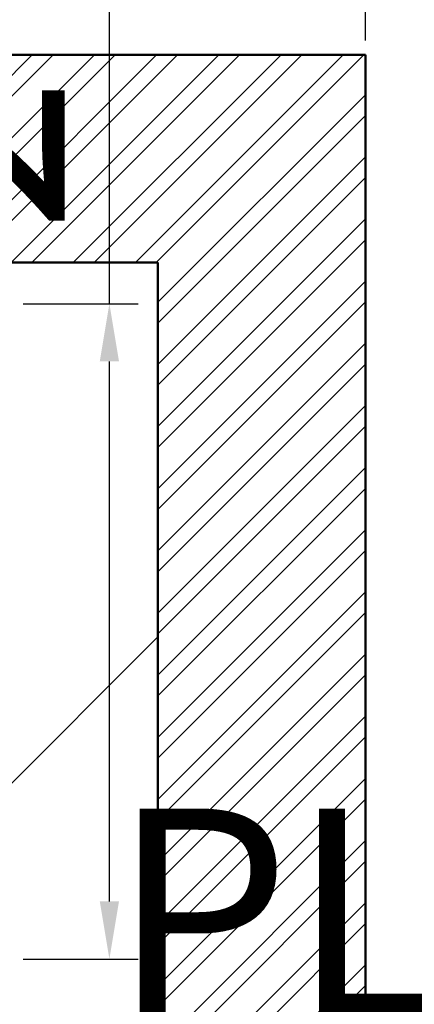
# Model space of a CAD drawing. Units: inches. Extents: x 3590 to 5167, y 65 to 1917.
# Tile 98 of 100: x 5065 to 5082, y 1765 to 1808. Entities that reach past the tile are written whole.
import ezdxf

# ---------------------------------------------------------------- set-up
doc = ezdxf.new("R2010")
doc.units = ezdxf.units.IN
for name, color, linetype, lineweight in [('A-ANNO-DIMS', 2, 'Continuous', 18), ('A-FLOR-PATT', 8, 'Continuous', 13), ('A-WALL', 7, 'Continuous', 50), ('A-WALL-PATT', 251, 'Continuous', 13)]:
    doc.layers.add(name, color=color, linetype=linetype, lineweight=lineweight)
doc.styles.get("Standard").update_dxf_attribs({"font": 'arial.ttf'})
doc.dimstyles.new('ISO-25', dxfattribs={"dimtxt": 9, "dimasz": 2.5, "dimexe": 1.25, "dimexo": 0.625, "dimtad": 1, "dimdec": 1, "dimlunit": 3, "dimtxsty": 'Standard', "dimcen": 2.5, "dimadec": 0, "dimazin": 0, "dimtfac": 1, "dimtdec": 1, "dimtmove": 0, "dimatfit": 3, "dimfxl": 1, "dimarcsym": 0})

# ---------------------------------------------------------------- blocks, each defined once
blk = doc.blocks.new('*D101')
at = {"layer": 'A-ANNO-DIMS', "color": 0, "lineweight": -2, "transparency": 16777216}
for p, q in [((4420.274, 1806.624), (4420.274, 1818.615)), ((5080.274, 1806.624), (5080.274, 1818.615)), ((4422.774, 1817.365), (5077.774, 1817.365))]:
    blk.add_line(p, q, dxfattribs=at)
at = {"layer": 'A-ANNO-DIMS', "color": 0, "transparency": 16777216}
for points in [[(4422.774, 1817.781), (4422.774, 1816.948), (4420.274, 1817.365)], [(5077.774, 1817.781), (5077.774, 1816.948), (5080.274, 1817.365)]]:
    blk.add_solid(points, dxfattribs=at)
at = {"layer": 'Defpoints', "color": 0, "transparency": 16777216}
for p in [(5080.274, 1817.365), (4420.274, 1805.999), (5080.274, 1805.999)]:
    blk.add_point(p, dxfattribs=at)
at = {"layer": 'A-ANNO-DIMS', "color": 0, "transparency": 16777216, "insert": (4750.274, 1822.566), "char_height": 9, "attachment_point": 5}
blk.add_mtext("55'", dxfattribs=at)
blk = doc.blocks.new('*D322')
at = {"layer": 'A-ANNO-DIMS', "color": 0, "lineweight": -2, "transparency": 16777216}
for p, q in [((5035.744, 1766.184), (5035.744, 1761.199)), ((5064.812, 1766.184), (5064.812, 1761.199)), ((5038.244, 1762.449), (5062.312, 1762.449)), ((5064.812, 1762.449), (5166.991, 1762.449))]:
    blk.add_line(p, q, dxfattribs=at)
at = {"layer": 'A-ANNO-DIMS', "color": 0, "transparency": 16777216}
for points in [[(5038.244, 1762.866), (5038.244, 1762.032), (5035.744, 1762.449)], [(5062.312, 1762.866), (5062.312, 1762.032), (5064.812, 1762.449)]]:
    blk.add_solid(points, dxfattribs=at)
at = {"layer": 'Defpoints', "color": 0, "transparency": 16777216}
for p in [(5035.744, 1766.809), (5064.812, 1766.809), (5064.812, 1762.449)]:
    blk.add_point(p, dxfattribs=at)
at = {"layer": 'A-ANNO-DIMS', "color": 0, "transparency": 16777216, "insert": (5117.152, 1767.669), "char_height": 9, "attachment_point": 5}
blk.add_mtext('PLANT 2\'-5" TYP.', dxfattribs=at)
blk = doc.blocks.new('*D323')
at = {"layer": 'A-ANNO-DIMS', "color": 0, "lineweight": -2, "transparency": 16777216}
for p, q in [((5069.172, 1795.216), (5069.172, 1874.95)), ((5065.437, 1795.216), (5070.422, 1795.216)), ((5069.172, 1769.309), (5069.172, 1792.716)), ((5065.437, 1766.809), (5070.422, 1766.809))]:
    blk.add_line(p, q, dxfattribs=at)
at = {"layer": 'A-ANNO-DIMS', "color": 0, "transparency": 16777216}
for points in [[(5068.756, 1792.716), (5069.589, 1792.716), (5069.172, 1795.216)], [(5068.756, 1769.309), (5069.589, 1769.309), (5069.172, 1766.809)]]:
    blk.add_solid(points, dxfattribs=at)
at = {"layer": 'Defpoints', "color": 0, "transparency": 16777216}
for p in [(5064.812, 1795.216), (5069.172, 1795.216), (5064.812, 1766.809)]:
    blk.add_point(p, dxfattribs=at)
at = {"layer": 'A-ANNO-DIMS', "color": 0, "transparency": 16777216, "insert": (5063.894, 1836.333), "char_height": 9, "attachment_point": 5, "rotation": 90}
blk.add_mtext('2\'-4 1/2" TYP.', dxfattribs=at)

msp = doc.modelspace()

# ---------------------------------------------------------------- hatches: boundary and pattern name
at = {"layer": 'A-FLOR-PATT', "transparency": 33554687}
h = msp.add_hatch(dxfattribs=at)
h.set_pattern_fill('AR-HBONE', color=256, scale=0.2)
h.set_pattern_definition([(45, (-588.972, 0), (0, 28.73682), [60.96, -20.32]), (135, (-574.604, 14.368), (3e-15, 28.73682), [60.96, -20.32])])
h.paths.add_polyline_path([(5071.274, 1796.999), (4933.274, 1796.999), (4933.274, 1753.999), (4962.774, 1753.999, -0.414214), (4928.774, 1719.999), (4933.274, 1718.999), (4933.274, 1334.999), (5071.274, 1334.999)])
h.paths.add_polyline_path([(4951.78, 1521.077), (4951.715, 1521.04), (4951.563, 1520.895)], flags=16)
h.paths.add_polyline_path([(4952.267, 1521.376), (4952.198, 1521.371), (4952.198, 1521.356)], flags=0)
h.paths.add_polyline_path([(4967.051, 1529.728), (4965.231, 1528.694), (4963.411, 1527.714), (4961.756, 1526.851), (4963.589, 1527.449), (4964.036, 1527.478), (4962.975, 1527.249), (4961.76, 1526.852), (4959.792, 1525.834), (4958.005, 1524.895), (4956.24, 1523.93), (4954.504, 1522.919), (4954.129, 1522.682), (4953.361, 1521.997), (4953.366, 1521.998), (4953.605, 1522.064), (4955.106, 1522.761), (4956.921, 1523.434), (4958.678, 1523.915), (4960.358, 1524.2), (4961.945, 1524.286), (4964.171, 1524.108), (4965.958, 1523.309), (4963.863, 1522.976), (4965.187, 1522.499), (4963.366, 1522.497), (4961.545, 1522.487), (4959.764, 1522.461), (4958.304, 1522.419), (4957.974, 1522.388), (4956.307, 1522.232), (4954.718, 1522.071), (4953.251, 1521.899), (4953.525, 1521.623), (4954.331, 1521.379), (4956.243, 1521.23), (4958.039, 1520.93), (4959.684, 1520.483), (4961.16, 1519.896), (4963.107, 1518.8), (4964.393, 1517.325), (4962.973, 1517.726), (4964.558, 1516.661), (4965.407, 1515.708), (4963.507, 1516.322), (4961.68, 1517.005), (4959.935, 1517.745), (4958.282, 1518.528), (4956.732, 1519.343), (4955.295, 1520.175), (4954.672, 1520.572), (4954.513, 1520.627), (4955.658, 1519.318), (4956.703, 1517.982), (4957.644, 1516.647), (4958.485, 1515.334), (4959.55, 1513.524), (4960.438, 1511.769), (4958.841, 1513.62), (4957.452, 1515.325), (4955.819, 1517.459), (4956.665, 1515.448), (4957.111, 1513.923), (4957.447, 1511.714), (4957.076, 1509.793), (4956.538, 1511.11), (4955.992, 1512.569), (4955.444, 1514.125), (4954.898, 1515.735), (4954.357, 1517.356), (4953.824, 1518.943), (4953.305, 1520.452), (4953.065, 1521.116), (4952.971, 1521.146), (4952.949, 1521.086), (4952.73, 1520.199), (4953.37, 1518.024), (4953.757, 1516.373), (4954.051, 1514.765), (4954.264, 1513.221), (4954.471, 1511.131), (4954.497, 1510.402), (4954.409, 1511.76), (4954.264, 1513.221), (4954.051, 1514.765), (4953.757, 1516.373), (4953.37, 1518.024), (4952.877, 1519.698), (4952.716, 1520.141), (4952.533, 1519.059), (4952.374, 1517.789), (4952.219, 1516.312), (4952.046, 1514.6), (4951.833, 1512.626), (4951.557, 1510.363), (4951.203, 1512.168), (4950.852, 1514.339), (4950.985, 1516.376), (4951.66, 1518.286), (4952.593, 1520.481), (4952.357, 1521.13), (4951.855, 1520.328), (4950.839, 1518.908), (4949.777, 1517.587), (4948.916, 1516.617), (4948.111, 1515.256), (4947.089, 1513.554), (4945.889, 1511.615), (4946.326, 1513.402), (4946.562, 1514.249), (4945.528, 1513.327), (4944.581, 1512.531), (4946.018, 1514.508), (4947.204, 1516.048), (4947.893, 1517.313), (4949.307, 1518.764), (4950.414, 1519.767), (4950.451, 1519.806), (4952.267, 1521.376), (4951.645, 1521.493), (4950.404, 1521.18), (4948.044, 1520.359), (4946.119, 1519.452), (4944.572, 1518.475), (4943.35, 1517.443), (4941.997, 1515.92), (4941.661, 1515.275), (4942.813, 1516.99), (4944.572, 1518.475), (4946.119, 1519.452), (4948.044, 1520.359), (4950.404, 1521.18), (4951.645, 1521.493), (4949.647, 1521.868), (4948.6, 1521.756), (4947.126, 1521.57), (4945.42, 1521.348), (4943.45, 1521.105), (4941.183, 1520.856), (4942.86, 1521.613), (4943.873, 1522.03), (4942.952, 1521.909), (4941.41, 1521.485), (4939.543, 1520.67), (4938.968, 1520.226), (4940.733, 1521.299), (4942.952, 1521.909), (4943.702, 1522.008), (4945.894, 1522.7), (4947.565, 1522.714), (4948.921, 1522.566), (4951.131, 1522.183), (4950.971, 1522.297), (4948.129, 1523.006), (4946.035, 1523.707), (4944.232, 1524.521), (4942.707, 1525.461), (4941.444, 1526.537), (4940.43, 1527.761), (4939.649, 1529.143), (4941.421, 1528.122), (4943.147, 1527.132), (4944.841, 1526.175), (4946.514, 1525.25), (4948.179, 1524.359), (4948.365, 1524.263), (4946.475, 1526.045), (4945.181, 1527.54), (4944.19, 1529.033), (4943.496, 1530.54), (4943.278, 1531.36), (4942.498, 1531.919), (4943.114, 1531.762), (4942.959, 1533.659), (4944.14, 1531.989), (4944.612, 1531.323), (4946.202, 1530.463), (4947.486, 1529.509), (4948.79, 1528.226), (4950.368, 1526.237), (4949.485, 1528.155), (4948.851, 1530.123), (4948.491, 1532.041), (4948.381, 1533.918), (4948.501, 1535.76), (4948.827, 1537.573), (4949.418, 1535.565), (4949.957, 1533.569), (4950.464, 1531.586), (4950.961, 1529.617), (4951.391, 1527.954), (4951.724, 1530.687), (4952.201, 1532.58), (4952.889, 1534.33), (4953.77, 1535.951), (4954.827, 1537.46), (4954.521, 1535.39), (4954.273, 1533.937), (4955.58, 1535.663), (4956.748, 1536.739), (4956.159, 1534.78), (4955.589, 1532.873), (4955.043, 1531.006), (4954.525, 1529.166), (4954.038, 1527.341), (4953.638, 1525.733), (4953.611, 1525.586), (4953.398, 1524.166), (4953.382, 1524.009), (4954.07, 1525.476), (4954.912, 1527.022), (4956.136, 1528.894), (4957.847, 1530.577), (4959.376, 1531.54), (4958.256, 1530.104), (4957.143, 1528.663), (4956.066, 1527.243), (4955.056, 1525.871), (4954.141, 1524.571), (4953.352, 1523.372), (4953.311, 1523.303), (4953.273, 1522.925), (4953.261, 1522.382), (4954.103, 1523.373), (4954.63, 1524.284), (4955.961, 1526.358), (4957.23, 1528.13), (4958.421, 1529.609), (4960.037, 1531.368), (4961.374, 1532.375), (4962.101, 1532.77), (4961.07, 1531.061), (4959.987, 1529.438), (4958.869, 1527.908), (4958.15, 1527.007), (4959.803, 1528.003), (4961.589, 1528.793), (4963.391, 1529.328), (4965.211, 1529.632)], flags=16)
h.paths.add_polyline_path([(4962.944, 1523.182), (4961.107, 1523.422), (4960.392, 1523.362), (4962.35, 1523.331)], flags=0)
h.paths.add_polyline_path([(5049.541, 1584.551), (5049.476, 1584.515), (5049.325, 1584.37)], flags=16)
h.paths.add_polyline_path([(5050.028, 1584.851), (5049.959, 1584.845), (5049.959, 1584.83)], flags=0)
h.paths.add_polyline_path([(5042.333, 1581.949), (5043.88, 1582.926), (5045.806, 1583.833), (5048.165, 1584.654), (5049.406, 1584.967), (5047.408, 1585.342), (5046.361, 1585.231), (5044.888, 1585.044), (5043.181, 1584.822), (5041.211, 1584.579), (5038.944, 1584.33), (5040.622, 1585.087), (5041.634, 1585.504), (5040.713, 1585.383), (5039.171, 1584.959), (5037.304, 1584.144), (5036.729, 1583.7), (5038.494, 1584.773), (5040.713, 1585.383), (5041.463, 1585.482), (5043.655, 1586.174), (5045.326, 1586.188), (5046.682, 1586.04), (5048.893, 1585.657), (5048.732, 1585.771), (5045.891, 1586.48), (5043.796, 1587.181), (5041.994, 1587.996), (5040.468, 1588.935), (5039.205, 1590.011), (5038.191, 1591.235), (5037.41, 1592.617), (5039.182, 1591.596), (5040.909, 1590.607), (5042.602, 1589.649), (5044.275, 1588.724), (5045.94, 1587.833), (5046.126, 1587.738), (5044.237, 1589.519), (5042.942, 1591.015), (5041.952, 1592.508), (5041.257, 1594.014), (5041.039, 1594.834), (5040.26, 1595.393), (5040.875, 1595.237), (5040.721, 1597.133), (5041.901, 1595.463), (5042.373, 1594.798), (5043.963, 1593.938), (5045.247, 1592.983), (5046.552, 1591.701), (5048.129, 1589.712), (5047.247, 1591.63), (5046.613, 1593.597), (5046.252, 1595.515), (5046.142, 1597.392), (5046.262, 1599.234), (5046.588, 1601.047), (5047.179, 1599.039), (5047.718, 1597.043), (5048.225, 1595.06), (5048.722, 1593.091), (5049.152, 1591.429), (5049.485, 1594.161), (5049.962, 1596.054), (5050.65, 1597.804), (5051.532, 1599.425), (5052.589, 1600.934), (5052.283, 1598.864), (5052.034, 1597.411), (5053.341, 1599.137), (5054.509, 1600.213), (5053.92, 1598.254), (5053.35, 1596.348), (5052.805, 1594.48), (5052.286, 1592.64), (5051.799, 1590.815), (5051.4, 1589.207), (5051.373, 1589.06), (5051.159, 1587.64), (5051.143, 1587.483), (5051.831, 1588.95), (5052.673, 1590.496), (5053.898, 1592.368), (5055.608, 1594.051), (5057.137, 1595.014), (5056.017, 1593.578), (5054.904, 1592.137), (5053.828, 1590.717), (5052.817, 1589.345), (5051.902, 1588.046), (5051.113, 1586.846), (5051.072, 1586.777), (5051.034, 1586.399), (5051.022, 1585.856), (5051.864, 1586.847), (5052.391, 1587.758), (5053.723, 1589.832), (5054.991, 1591.604), (5056.182, 1593.083), (5057.798, 1594.842), (5059.135, 1595.849), (5059.863, 1596.244), (5058.831, 1594.535), (5057.749, 1592.912), (5056.63, 1591.382), (5055.912, 1590.482), (5057.564, 1591.477), (5059.35, 1592.267), (5061.152, 1592.802), (5062.972, 1593.106), (5064.812, 1593.203), (5062.992, 1592.169), (5061.172, 1591.188), (5059.518, 1590.325), (5061.35, 1590.924), (5061.797, 1590.952), (5060.737, 1590.723), (5059.521, 1590.326), (5057.553, 1589.308), (5055.766, 1588.369), (5054.002, 1587.404), (5052.265, 1586.393), (5051.891, 1586.156), (5051.122, 1585.471), (5051.127, 1585.472), (5051.366, 1585.538), (5052.867, 1586.235), (5054.682, 1586.908), (5056.439, 1587.389), (5058.12, 1587.675), (5059.706, 1587.76), (5061.933, 1587.583), (5063.719, 1586.783), (5061.624, 1586.45), (5062.949, 1585.973), (5061.127, 1585.971), (5059.307, 1585.961), (5057.525, 1585.935), (5056.065, 1585.893), (5055.735, 1585.862), (5054.068, 1585.707), (5052.479, 1585.546), (5051.012, 1585.373), (5051.286, 1585.097), (5052.092, 1584.853), (5054.004, 1584.704), (5055.8, 1584.404), (5057.446, 1583.958), (5058.921, 1583.37), (5060.868, 1582.274), (5062.154, 1580.799), (5060.734, 1581.2), (5062.32, 1580.135), (5063.168, 1579.182), (5061.269, 1579.796), (5059.441, 1580.479), (5057.696, 1581.219), (5056.043, 1582.003), (5054.493, 1582.817), (5053.057, 1583.649), (5052.433, 1584.047), (5052.274, 1584.101), (5053.42, 1582.793), (5054.464, 1581.457), (5055.405, 1580.121), (5056.247, 1578.809), (5057.311, 1576.998), (5058.199, 1575.244), (5056.602, 1577.094), (5055.213, 1578.799), (5053.58, 1580.933), (5054.427, 1578.922), (5054.872, 1577.397), (5055.208, 1575.189), (5054.838, 1573.267), (5054.299, 1574.584), (5053.754, 1576.043), (5053.206, 1577.599), (5052.659, 1579.209), (5052.118, 1580.83), (5051.585, 1582.417), (5051.066, 1583.927), (5050.826, 1584.59), (5050.733, 1584.62), (5050.711, 1584.561), (5050.491, 1583.673), (5051.131, 1581.498), (5051.518, 1579.847), (5051.813, 1578.24), (5052.026, 1576.695), (5052.233, 1574.605), (5052.258, 1573.876), (5052.17, 1575.234), (5052.026, 1576.695), (5051.813, 1578.24), (5051.518, 1579.847), (5051.131, 1581.498), (5050.638, 1583.172), (5050.477, 1583.615), (5050.294, 1582.533), (5050.136, 1581.263), (5049.981, 1579.786), (5049.807, 1578.074), (5049.594, 1576.1), (5049.318, 1573.837), (5048.965, 1575.642), (5048.613, 1577.813), (5048.747, 1579.85), (5049.421, 1581.76), (5050.354, 1583.955), (5050.118, 1584.604), (5049.616, 1583.802), (5048.6, 1582.382), (5047.538, 1581.061), (5046.677, 1580.091), (5045.872, 1578.73), (5044.85, 1577.028), (5043.651, 1575.089), (5044.087, 1576.877), (5044.324, 1577.723), (5043.289, 1576.801), (5042.342, 1576.005), (5043.779, 1577.982), (5044.966, 1579.522), (5045.655, 1580.787), (5047.068, 1582.239), (5048.175, 1583.241), (5048.213, 1583.28), (5050.028, 1584.851), (5049.406, 1584.967), (5048.165, 1584.654), (5045.806, 1583.833), (5043.88, 1582.926), (5042.333, 1581.949), (5041.111, 1580.917), (5039.758, 1579.394), (5039.423, 1578.749), (5040.575, 1580.464)], flags=16)
h.paths.add_polyline_path([(4954.799, 1533.12), (4954.262, 1532.079), (4953.831, 1530.935), (4953.505, 1529.636), (4953.283, 1528.133), (4953.167, 1526.376), (4953.156, 1524.315), (4953.277, 1521.236), (4952.802, 1521.842), (4951.557, 1521.998), (4950.976, 1521.961), (4952.661, 1521.941), (4952.802, 1521.842), (4953.152, 1523.593), (4953.167, 1526.376), (4953.283, 1528.133), (4953.609, 1530.346), (4954.456, 1532.592)], flags=0)
h.paths.add_polyline_path([(5050.563, 1585.316), (5049.318, 1585.472), (5048.737, 1585.435), (5050.422, 1585.415), (5050.563, 1585.316), (5050.914, 1587.067), (5050.928, 1589.851), (5051.045, 1591.607), (5051.371, 1593.82), (5052.217, 1596.066), (5052.56, 1596.594), (5052.024, 1595.554), (5051.592, 1594.409), (5051.266, 1593.11), (5051.045, 1591.607), (5050.928, 1589.851), (5050.918, 1587.789), (5051.038, 1584.71)], flags=0)
h.paths.add_polyline_path([(5058.153, 1586.836), (5060.111, 1586.805), (5060.705, 1586.656), (5058.868, 1586.896)], flags=0)
h.paths.add_polyline_path([(5049.541, 1430.936), (5049.476, 1430.9), (5049.325, 1430.755)], flags=16)
h.paths.add_polyline_path([(5050.028, 1431.236), (5049.959, 1431.231), (5049.959, 1431.215)], flags=0)
h.paths.add_polyline_path([(5046.588, 1447.432), (5047.179, 1445.425), (5047.718, 1443.429), (5048.225, 1441.446), (5048.722, 1439.476), (5049.152, 1437.814), (5049.485, 1440.546), (5049.962, 1442.439), (5050.65, 1444.189), (5051.532, 1445.811), (5052.589, 1447.319), (5052.283, 1445.249), (5052.034, 1443.796), (5053.341, 1445.522), (5054.509, 1446.598), (5053.92, 1444.64), (5053.35, 1442.733), (5052.805, 1440.865), (5052.286, 1439.025), (5051.799, 1437.201), (5051.4, 1435.592), (5051.373, 1435.445), (5051.159, 1434.025), (5051.143, 1433.868), (5051.831, 1435.335), (5052.673, 1436.881), (5053.898, 1438.753), (5055.608, 1440.436), (5057.137, 1441.4), (5056.017, 1439.963), (5054.904, 1438.522), (5053.828, 1437.102), (5052.817, 1435.73), (5051.902, 1434.431), (5051.113, 1433.231), (5051.072, 1433.162), (5051.034, 1432.784), (5051.022, 1432.242), (5051.864, 1433.232), (5052.391, 1434.143), (5053.723, 1436.217), (5054.991, 1437.989), (5056.182, 1439.468), (5057.798, 1441.227), (5059.135, 1442.235), (5059.863, 1442.629), (5058.831, 1440.921), (5057.749, 1439.298), (5056.63, 1437.767), (5055.912, 1436.867), (5057.564, 1437.863), (5059.35, 1438.652), (5061.152, 1439.187), (5062.972, 1439.491), (5064.812, 1439.588), (5062.992, 1438.554), (5061.172, 1437.573), (5059.518, 1436.71), (5061.35, 1437.309), (5061.797, 1437.337), (5060.737, 1437.108), (5059.521, 1436.711), (5057.553, 1435.693), (5055.766, 1434.754), (5054.002, 1433.789), (5052.265, 1432.778), (5051.891, 1432.541), (5051.122, 1431.856), (5051.127, 1431.857), (5051.366, 1431.923), (5052.867, 1432.62), (5054.682, 1433.293), (5056.439, 1433.775), (5058.12, 1434.06), (5059.706, 1434.145), (5061.933, 1433.968), (5063.719, 1433.168), (5061.624, 1432.835), (5062.949, 1432.358), (5061.127, 1432.357), (5059.307, 1432.346), (5057.525, 1432.32), (5056.065, 1432.278), (5055.735, 1432.248), (5054.068, 1432.092), (5052.479, 1431.931), (5051.012, 1431.759), (5051.286, 1431.482), (5052.092, 1431.238), (5054.004, 1431.089), (5055.8, 1430.789), (5057.446, 1430.343), (5058.921, 1429.755), (5060.868, 1428.66), (5062.154, 1427.185), (5060.734, 1427.585), (5062.32, 1426.52), (5063.168, 1425.567), (5061.269, 1426.181), (5059.441, 1426.865), (5057.696, 1427.604), (5056.043, 1428.388), (5054.493, 1429.202), (5053.057, 1430.034), (5052.433, 1430.432), (5052.274, 1430.487), (5053.42, 1429.178), (5054.464, 1427.842), (5055.405, 1426.506), (5056.247, 1425.194), (5057.311, 1423.383), (5058.199, 1421.629), (5056.602, 1423.479), (5055.213, 1425.184), (5053.58, 1427.318), (5054.427, 1425.307), (5054.872, 1423.782), (5055.208, 1421.574), (5054.838, 1419.652), (5054.299, 1420.97), (5053.754, 1422.428), (5053.206, 1423.984), (5052.659, 1425.595), (5052.118, 1427.215), (5051.585, 1428.802), (5051.066, 1430.312), (5050.826, 1430.975), (5050.733, 1431.005), (5050.711, 1430.946), (5050.491, 1430.058), (5051.131, 1427.883), (5051.518, 1426.232), (5051.813, 1424.625), (5052.026, 1423.081), (5052.233, 1420.991), (5052.258, 1420.261), (5052.17, 1421.619), (5052.026, 1423.081), (5051.813, 1424.625), (5051.518, 1426.232), (5051.131, 1427.883), (5050.638, 1429.558), (5050.477, 1430.001), (5050.294, 1428.918), (5050.136, 1427.648), (5049.981, 1426.171), (5049.807, 1424.459), (5049.594, 1422.485), (5049.318, 1420.222), (5048.965, 1422.028), (5048.613, 1424.199), (5048.747, 1426.235), (5049.421, 1428.146), (5050.354, 1430.34), (5050.118, 1430.989), (5049.616, 1430.187), (5048.6, 1428.768), (5047.538, 1427.446), (5046.677, 1426.477), (5045.872, 1425.116), (5044.85, 1423.413), (5043.651, 1421.474), (5044.087, 1423.262), (5044.324, 1424.109), (5043.289, 1423.186), (5042.342, 1422.391), (5043.779, 1424.368), (5044.966, 1425.907), (5045.655, 1427.173), (5047.068, 1428.624), (5048.175, 1429.627), (5048.213, 1429.666), (5050.028, 1431.236), (5049.406, 1431.353), (5048.165, 1431.039), (5045.806, 1430.218), (5043.88, 1429.311), (5042.333, 1428.334), (5041.111, 1427.302), (5039.758, 1425.779), (5039.423, 1425.134), (5040.575, 1426.849), (5042.333, 1428.334), (5043.88, 1429.311), (5045.806, 1430.218), (5048.165, 1431.039), (5049.406, 1431.353), (5047.408, 1431.727), (5046.361, 1431.616), (5044.888, 1431.429), (5043.181, 1431.207), (5041.211, 1430.964), (5038.944, 1430.715), (5040.622, 1431.472), (5041.634, 1431.89), (5040.713, 1431.769), (5039.171, 1431.345), (5037.304, 1430.53), (5036.729, 1430.085), (5038.494, 1431.158), (5040.713, 1431.769), (5041.463, 1431.867), (5043.655, 1432.559), (5045.326, 1432.573), (5046.682, 1432.425), (5048.893, 1432.042), (5048.732, 1432.156), (5045.891, 1432.865), (5043.796, 1433.566), (5041.994, 1434.381), (5040.468, 1435.321), (5039.205, 1436.396), (5038.191, 1437.62), (5037.41, 1439.002), (5039.182, 1437.982), (5040.909, 1436.992), (5042.602, 1436.034), (5044.275, 1435.109), (5045.94, 1434.218), (5046.126, 1434.123), (5044.237, 1435.904), (5042.942, 1437.4), (5041.952, 1438.893), (5041.257, 1440.399), (5041.039, 1441.219), (5040.26, 1441.778), (5040.875, 1441.622), (5040.721, 1443.518), (5041.901, 1441.848), (5042.373, 1441.183), (5043.963, 1440.323), (5045.247, 1439.369), (5046.552, 1438.086), (5048.129, 1436.097), (5047.247, 1438.015), (5046.613, 1439.982), (5046.252, 1441.901), (5046.142, 1443.778), (5046.262, 1445.619)], flags=16)
h.paths.add_polyline_path([(5052.382, 1444.255), (5051.623, 1442.78), (5052.024, 1441.939), (5052.56, 1442.98)], flags=0)
h.paths.add_polyline_path([(5050.563, 1431.701), (5049.318, 1431.857), (5048.737, 1431.821), (5050.422, 1431.8)], flags=0)
h.paths.add_polyline_path([(5058.153, 1433.221), (5060.111, 1433.19), (5060.705, 1433.041), (5058.868, 1433.281)], flags=0)
h.paths.add_polyline_path([(5049.541, 1352.285), (5049.476, 1352.249), (5049.325, 1352.104)], flags=16)
h.paths.add_polyline_path([(5050.028, 1352.585), (5049.959, 1352.58), (5049.959, 1352.564)], flags=0)
h.paths.add_polyline_path([(5046.588, 1368.781), (5047.179, 1366.774), (5047.718, 1364.778), (5048.225, 1362.795), (5048.722, 1360.825), (5049.152, 1359.163), (5049.485, 1361.896), (5049.962, 1363.789), (5050.65, 1365.538), (5051.532, 1367.16), (5052.589, 1368.669), (5052.283, 1366.598), (5052.034, 1365.145), (5053.341, 1366.871), (5054.509, 1367.947), (5053.92, 1365.989), (5053.35, 1364.082), (5052.805, 1362.214), (5052.286, 1360.374), (5051.799, 1358.55), (5051.4, 1356.942), (5051.373, 1356.794), (5051.159, 1355.374), (5051.143, 1355.218), (5051.831, 1356.684), (5052.673, 1358.23), (5053.898, 1360.102), (5055.608, 1361.786), (5057.137, 1362.749), (5056.017, 1361.313), (5054.904, 1359.872), (5053.828, 1358.452), (5052.817, 1357.079), (5051.902, 1355.78), (5051.113, 1354.581), (5051.072, 1354.512), (5051.034, 1354.133), (5051.022, 1353.591), (5051.864, 1354.581), (5052.391, 1355.492), (5053.723, 1357.566), (5054.991, 1359.338), (5056.182, 1360.817), (5057.798, 1362.577), (5059.135, 1363.584), (5059.863, 1363.979), (5058.831, 1362.27), (5057.749, 1360.647), (5056.63, 1359.117), (5055.912, 1358.216), (5057.564, 1359.212), (5059.35, 1360.001), (5061.152, 1360.536), (5062.972, 1360.841), (5064.812, 1360.937), (5062.992, 1359.903), (5061.172, 1358.923), (5059.518, 1358.059), (5061.35, 1358.658), (5061.797, 1358.687), (5060.737, 1358.458), (5059.521, 1358.061), (5057.553, 1357.043), (5055.766, 1356.103), (5054.002, 1355.138), (5052.265, 1354.127), (5051.891, 1353.89), (5051.122, 1353.206), (5051.127, 1353.206), (5051.366, 1353.272), (5052.867, 1353.969), (5054.682, 1354.643), (5056.439, 1355.124), (5058.12, 1355.409), (5059.706, 1355.495), (5061.933, 1355.317), (5063.719, 1354.518), (5061.624, 1354.184), (5062.949, 1353.708), (5061.127, 1353.706), (5059.307, 1353.695), (5057.525, 1353.669), (5056.065, 1353.627), (5055.735, 1353.597), (5054.068, 1353.441), (5052.479, 1353.28), (5051.012, 1353.108), (5051.286, 1352.831), (5052.092, 1352.587), (5054.004, 1352.439), (5055.8, 1352.138), (5057.446, 1351.692), (5058.921, 1351.104), (5060.868, 1350.009), (5062.154, 1348.534), (5060.734, 1348.935), (5062.32, 1347.869), (5063.168, 1346.916), (5061.269, 1347.53), (5059.441, 1348.214), (5057.696, 1348.954), (5056.043, 1349.737), (5054.493, 1350.551), (5053.057, 1351.383), (5052.433, 1351.781), (5052.274, 1351.836), (5053.42, 1350.527), (5054.464, 1349.191), (5055.405, 1347.855), (5056.247, 1346.543), (5057.311, 1344.733), (5058.199, 1342.978), (5056.602, 1344.828), (5055.213, 1346.534), (5053.58, 1348.667), (5054.427, 1346.656), (5054.872, 1345.132), (5055.208, 1342.923), (5054.838, 1341.002), (5054.299, 1342.319), (5053.754, 1343.778), (5053.206, 1345.334), (5052.659, 1346.944), (5052.118, 1348.564), (5051.585, 1350.151), (5051.066, 1351.661), (5050.826, 1352.324), (5050.733, 1352.355), (5050.711, 1352.295), (5050.491, 1351.408), (5051.131, 1349.232), (5051.518, 1347.581), (5051.813, 1345.974), (5052.026, 1344.43), (5052.233, 1342.34), (5052.258, 1341.61), (5052.17, 1342.969), (5052.026, 1344.43), (5051.813, 1345.974), (5051.518, 1347.581), (5051.131, 1349.232), (5050.638, 1350.907), (5050.477, 1351.35), (5050.294, 1350.267), (5050.136, 1348.997), (5049.981, 1347.52), (5049.807, 1345.809), (5049.594, 1343.835), (5049.318, 1341.571), (5048.965, 1343.377), (5048.613, 1345.548), (5048.747, 1347.585), (5049.421, 1349.495), (5050.354, 1351.689), (5050.118, 1352.339), (5049.616, 1351.536), (5048.6, 1350.117), (5047.538, 1348.795), (5046.677, 1347.826), (5045.872, 1346.465), (5044.85, 1344.763), (5043.651, 1342.824), (5044.087, 1344.611), (5044.324, 1345.458), (5043.289, 1344.535), (5042.342, 1343.74), (5043.779, 1345.717), (5044.966, 1347.256), (5045.655, 1348.522), (5047.068, 1349.973), (5048.175, 1350.976), (5048.213, 1351.015), (5050.028, 1352.585), (5049.406, 1352.702), (5048.165, 1352.388), (5045.806, 1351.567), (5043.88, 1350.661), (5042.333, 1349.683), (5041.111, 1348.651), (5039.758, 1347.128), (5039.423, 1346.483), (5040.575, 1348.198), (5042.333, 1349.683), (5043.88, 1350.661), (5045.806, 1351.567), (5048.165, 1352.388), (5049.406, 1352.702), (5047.408, 1353.076), (5046.361, 1352.965), (5044.888, 1352.779), (5043.181, 1352.556), (5041.211, 1352.313), (5038.944, 1352.065), (5040.622, 1352.821), (5041.634, 1353.239), (5040.713, 1353.118), (5039.171, 1352.694), (5037.304, 1351.879), (5036.729, 1351.434), (5038.494, 1352.508), (5040.713, 1353.118), (5041.463, 1353.216), (5043.655, 1353.909), (5045.326, 1353.923), (5046.682, 1353.774), (5048.893, 1353.391), (5048.732, 1353.506), (5045.891, 1354.214), (5043.796, 1354.915), (5041.994, 1355.73), (5040.468, 1356.67), (5039.205, 1357.746), (5038.191, 1358.969), (5037.41, 1360.352), (5039.182, 1359.331), (5040.909, 1358.341), (5042.602, 1357.383), (5044.275, 1356.458), (5045.94, 1355.567), (5046.126, 1355.472), (5044.237, 1357.253), (5042.942, 1358.749), (5041.952, 1360.242), (5041.257, 1361.748), (5041.039, 1362.568), (5040.26, 1363.128), (5040.875, 1362.971), (5040.721, 1364.867), (5041.901, 1363.197), (5042.373, 1362.532), (5043.963, 1361.672), (5045.247, 1360.718), (5046.552, 1359.435), (5048.129, 1357.446), (5047.247, 1359.364), (5046.613, 1361.331), (5046.252, 1363.25), (5046.142, 1365.127), (5046.262, 1366.969)], flags=16)
h.paths.add_polyline_path([(5052.382, 1365.604), (5051.623, 1364.129), (5052.024, 1363.288), (5052.56, 1364.329)], flags=0)
h.paths.add_polyline_path([(4951.78, 1698.041), (4951.715, 1698.005), (4951.563, 1697.859)], flags=16)
h.paths.add_polyline_path([(4952.267, 1698.341), (4952.198, 1698.335), (4952.198, 1698.32)], flags=0)
h.paths.add_polyline_path([(4957.076, 1686.757), (4956.538, 1688.074), (4955.992, 1689.533), (4955.444, 1691.089), (4954.898, 1692.699), (4954.357, 1694.32), (4953.824, 1695.907), (4953.305, 1697.417), (4953.065, 1698.08), (4952.971, 1698.11), (4952.949, 1698.051), (4952.73, 1697.163), (4953.37, 1694.988), (4953.757, 1693.337), (4954.051, 1691.729), (4954.264, 1690.185), (4954.471, 1688.095), (4954.497, 1687.366), (4954.409, 1688.724), (4954.264, 1690.185), (4954.051, 1691.729), (4953.757, 1693.337), (4953.37, 1694.988), (4952.877, 1696.662), (4952.716, 1697.105), (4952.533, 1696.023), (4952.374, 1694.753), (4952.219, 1693.276), (4952.046, 1691.564), (4951.833, 1689.59), (4951.557, 1687.327), (4951.203, 1689.132), (4950.852, 1691.303), (4950.985, 1693.34), (4951.66, 1695.25), (4952.593, 1697.445), (4952.357, 1698.094), (4951.855, 1697.292), (4950.839, 1695.872), (4949.777, 1694.551), (4948.916, 1693.581), (4948.111, 1692.22), (4947.089, 1690.518), (4945.889, 1688.579), (4946.326, 1690.366), (4946.562, 1691.213), (4945.528, 1690.291), (4944.581, 1689.495), (4946.018, 1691.472), (4947.204, 1693.012), (4947.893, 1694.277), (4949.307, 1695.729), (4950.414, 1696.731), (4950.451, 1696.77), (4952.267, 1698.341), (4951.645, 1698.457), (4950.404, 1698.144), (4948.044, 1697.323), (4946.119, 1696.416), (4944.572, 1695.439), (4943.35, 1694.407), (4941.997, 1692.884), (4941.661, 1692.239), (4942.813, 1693.954), (4944.572, 1695.439), (4946.119, 1696.416), (4948.044, 1697.323), (4950.404, 1698.144), (4951.645, 1698.457), (4949.647, 1698.832), (4948.6, 1698.72), (4947.126, 1698.534), (4945.42, 1698.312), (4943.45, 1698.069), (4941.183, 1697.82), (4942.86, 1698.577), (4943.873, 1698.994), (4942.952, 1698.873), (4941.41, 1698.449), (4939.543, 1697.634), (4938.968, 1697.19), (4940.733, 1698.263), (4942.952, 1698.873), (4943.702, 1698.972), (4945.894, 1699.664), (4947.565, 1699.678), (4948.921, 1699.53), (4951.131, 1699.147), (4950.971, 1699.261), (4948.129, 1699.97), (4946.035, 1700.671), (4944.232, 1701.486), (4942.707, 1702.425), (4941.444, 1703.501), (4940.43, 1704.725), (4939.649, 1706.107), (4941.421, 1705.086), (4943.147, 1704.097), (4944.841, 1703.139), (4946.514, 1702.214), (4948.179, 1701.323), (4948.365, 1701.227), (4946.475, 1703.009), (4945.181, 1704.505), (4944.19, 1705.997), (4943.496, 1707.504), (4943.278, 1708.324), (4942.498, 1708.883), (4943.114, 1708.727), (4942.959, 1710.623), (4944.14, 1708.953), (4944.612, 1708.287), (4946.202, 1707.428), (4947.486, 1706.473), (4948.79, 1705.191), (4950.368, 1703.202), (4949.485, 1705.12), (4948.851, 1707.087), (4948.491, 1709.005), (4948.381, 1710.882), (4948.501, 1712.724), (4948.827, 1714.537), (4949.418, 1712.529), (4949.957, 1710.533), (4950.464, 1708.55), (4950.961, 1706.581), (4951.391, 1704.919), (4951.724, 1707.651), (4952.201, 1709.544), (4952.889, 1711.294), (4953.77, 1712.915), (4954.827, 1714.424), (4954.521, 1712.354), (4954.273, 1710.901), (4955.58, 1712.627), (4956.748, 1713.703), (4956.159, 1711.744), (4955.589, 1709.837), (4955.043, 1707.97), (4954.525, 1706.13), (4954.038, 1704.305), (4953.638, 1702.697), (4953.611, 1702.55), (4953.398, 1701.13), (4953.382, 1700.973), (4954.07, 1702.44), (4954.912, 1703.986), (4956.136, 1705.858), (4957.847, 1707.541), (4959.376, 1708.504), (4958.256, 1707.068), (4957.143, 1705.627), (4956.066, 1704.207), (4955.056, 1702.835), (4954.141, 1701.536), (4953.352, 1700.336), (4953.311, 1700.267), (4953.273, 1699.889), (4953.261, 1699.346), (4954.103, 1700.337), (4954.63, 1701.248), (4955.961, 1703.322), (4957.23, 1705.094), (4958.421, 1706.573), (4960.037, 1708.332), (4961.374, 1709.339), (4962.101, 1709.734), (4961.07, 1708.025), (4959.987, 1706.402), (4958.869, 1704.872), (4958.15, 1703.972), (4959.803, 1704.967), (4961.589, 1705.757), (4963.391, 1706.292), (4965.211, 1706.596), (4967.051, 1706.692), (4965.231, 1705.659), (4963.411, 1704.678), (4961.756, 1703.815), (4963.589, 1704.413), (4964.036, 1704.442), (4962.975, 1704.213), (4961.76, 1703.816), (4959.792, 1702.798), (4958.005, 1701.859), (4956.24, 1700.894), (4954.504, 1699.883), (4954.129, 1699.646), (4953.361, 1698.961), (4953.366, 1698.962), (4953.605, 1699.028), (4955.106, 1699.725), (4956.921, 1700.398), (4958.678, 1700.879), (4960.358, 1701.164), (4961.945, 1701.25), (4964.171, 1701.073), (4965.958, 1700.273), (4963.863, 1699.94), (4965.187, 1699.463), (4963.366, 1699.461), (4961.545, 1699.451), (4959.764, 1699.425), (4958.304, 1699.383), (4957.974, 1699.352), (4956.307, 1699.197), (4954.718, 1699.036), (4953.251, 1698.863), (4953.525, 1698.587), (4954.331, 1698.343), (4956.243, 1698.194), (4958.039, 1697.894), (4959.684, 1697.447), (4961.16, 1696.86), (4963.107, 1695.764), (4964.393, 1694.289), (4962.973, 1694.69), (4964.558, 1693.625), (4965.407, 1692.672), (4963.507, 1693.286), (4961.68, 1693.969), (4959.935, 1694.709), (4958.282, 1695.492), (4956.732, 1696.307), (4955.295, 1697.139), (4954.672, 1697.536), (4954.513, 1697.591), (4955.658, 1696.282), (4956.703, 1694.946), (4957.644, 1693.611), (4958.485, 1692.298), (4959.55, 1690.488), (4960.438, 1688.733), (4958.841, 1690.584), (4957.452, 1692.289), (4955.819, 1694.423), (4956.665, 1692.412), (4957.111, 1690.887), (4957.447, 1688.678)], flags=16)
h.paths.add_polyline_path([(5050.563, 1353.05), (5049.318, 1353.207), (5048.737, 1353.17), (5050.422, 1353.15)], flags=0)
h.paths.add_polyline_path([(4951.78, 1351.486), (4951.715, 1351.45), (4951.563, 1351.305)], flags=16)
h.paths.add_polyline_path([(4952.267, 1351.786), (4952.198, 1351.78), (4952.198, 1351.765)], flags=0)
h.paths.add_polyline_path([(4954.827, 1367.869), (4954.521, 1365.799), (4954.273, 1364.346), (4955.58, 1366.072), (4956.748, 1367.148), (4956.159, 1365.19), (4955.589, 1363.283), (4955.043, 1361.415), (4954.525, 1359.575), (4954.038, 1357.751), (4953.638, 1356.142), (4953.611, 1355.995), (4953.398, 1354.575), (4953.382, 1354.418), (4954.07, 1355.885), (4954.912, 1357.431), (4956.136, 1359.303), (4957.847, 1360.986), (4959.376, 1361.95), (4958.256, 1360.513), (4957.143, 1359.072), (4956.066, 1357.652), (4955.056, 1356.28), (4954.141, 1354.981), (4953.352, 1353.781), (4953.311, 1353.712), (4953.273, 1353.334), (4953.261, 1352.792), (4954.103, 1353.782), (4954.63, 1354.693), (4955.961, 1356.767), (4957.23, 1358.539), (4958.421, 1360.018), (4960.037, 1361.777), (4961.374, 1362.785), (4962.101, 1363.179), (4961.07, 1361.471), (4959.987, 1359.848), (4958.869, 1358.317), (4958.15, 1357.417), (4959.803, 1358.413), (4961.589, 1359.202), (4963.391, 1359.737), (4965.211, 1360.041), (4967.051, 1360.138), (4965.231, 1359.104), (4963.411, 1358.123), (4961.756, 1357.26), (4963.589, 1357.859), (4964.036, 1357.887), (4962.975, 1357.658), (4961.76, 1357.261), (4959.792, 1356.243), (4958.005, 1355.304), (4956.24, 1354.339), (4954.504, 1353.328), (4954.129, 1353.091), (4953.361, 1352.406), (4953.366, 1352.407), (4953.605, 1352.473), (4955.106, 1353.17), (4956.921, 1353.843), (4958.678, 1354.325), (4960.358, 1354.61), (4961.945, 1354.695), (4964.171, 1354.518), (4965.958, 1353.718), (4963.863, 1353.385), (4965.187, 1352.908), (4963.366, 1352.907), (4961.545, 1352.896), (4959.764, 1352.87), (4958.304, 1352.828), (4957.974, 1352.798), (4956.307, 1352.642), (4954.718, 1352.481), (4953.251, 1352.309), (4953.525, 1352.032), (4954.331, 1351.788), (4956.243, 1351.639), (4958.039, 1351.339), (4959.684, 1350.893), (4961.16, 1350.305), (4963.107, 1349.21), (4964.393, 1347.735), (4962.973, 1348.135), (4964.558, 1347.07), (4965.407, 1346.117), (4963.507, 1346.731), (4961.68, 1347.414), (4959.935, 1348.154), (4958.282, 1348.938), (4956.732, 1349.752), (4955.295, 1350.584), (4954.672, 1350.982), (4954.513, 1351.036), (4955.658, 1349.728), (4956.703, 1348.392), (4957.644, 1347.056), (4958.485, 1345.744), (4959.55, 1343.933), (4960.438, 1342.179), (4958.841, 1344.029), (4957.452, 1345.734), (4955.819, 1347.868), (4956.665, 1345.857), (4957.111, 1344.332), (4957.447, 1342.124), (4957.076, 1340.202), (4956.538, 1341.52), (4955.992, 1342.978), (4955.444, 1344.534), (4954.898, 1346.145), (4954.357, 1347.765), (4953.824, 1349.352), (4953.305, 1350.862), (4953.065, 1351.525), (4952.971, 1351.555), (4952.949, 1351.496), (4952.73, 1350.608), (4953.37, 1348.433), (4953.757, 1346.782), (4954.051, 1345.175), (4954.264, 1343.631), (4954.471, 1341.541), (4954.497, 1340.811), (4954.409, 1342.169), (4954.264, 1343.631), (4954.051, 1345.175), (4953.757, 1346.782), (4953.37, 1348.433), (4952.877, 1350.108), (4952.716, 1350.551), (4952.533, 1349.468), (4952.374, 1348.198), (4952.219, 1346.721), (4952.046, 1345.009), (4951.833, 1343.035), (4951.557, 1340.772), (4951.203, 1342.578), (4950.852, 1344.749), (4950.985, 1346.785), (4951.66, 1348.696), (4952.593, 1350.89), (4952.357, 1351.539), (4951.855, 1350.737), (4950.839, 1349.318), (4949.777, 1347.996), (4948.916, 1347.027), (4948.111, 1345.665), (4947.089, 1343.963), (4945.889, 1342.024), (4946.326, 1343.812), (4946.562, 1344.659), (4945.528, 1343.736), (4944.581, 1342.941), (4946.018, 1344.918), (4947.204, 1346.457), (4947.893, 1347.723), (4949.307, 1349.174), (4950.414, 1350.177), (4950.451, 1350.216), (4952.267, 1351.786), (4951.645, 1351.903), (4950.404, 1351.589), (4948.044, 1350.768), (4946.119, 1349.861), (4944.572, 1348.884), (4943.35, 1347.852), (4941.997, 1346.329), (4941.661, 1345.684), (4942.813, 1347.399), (4944.572, 1348.884), (4946.119, 1349.861), (4948.044, 1350.768), (4950.404, 1351.589), (4951.645, 1351.903), (4949.647, 1352.277), (4948.6, 1352.166), (4947.126, 1351.979), (4945.42, 1351.757), (4943.45, 1351.514), (4941.183, 1351.265), (4942.86, 1352.022), (4943.873, 1352.44), (4942.952, 1352.319), (4941.41, 1351.895), (4939.543, 1351.08), (4938.968, 1350.635), (4940.733, 1351.708), (4942.952, 1352.319), (4943.702, 1352.417), (4945.894, 1353.109), (4947.565, 1353.123), (4948.921, 1352.975), (4951.131, 1352.592), (4950.971, 1352.706), (4948.129, 1353.415), (4946.035, 1354.116), (4944.232, 1354.931), (4942.707, 1355.871), (4941.444, 1356.946), (4940.43, 1358.17), (4939.649, 1359.552), (4941.421, 1358.532), (4943.147, 1357.542), (4944.841, 1356.584), (4946.514, 1355.659), (4948.179, 1354.768), (4948.365, 1354.673), (4946.475, 1356.454), (4945.181, 1357.95), (4944.19, 1359.443), (4943.496, 1360.949), (4943.278, 1361.769), (4942.498, 1362.328), (4943.114, 1362.172), (4942.959, 1364.068), (4944.14, 1362.398), (4944.612, 1361.733), (4946.202, 1360.873), (4947.486, 1359.919), (4948.79, 1358.636), (4950.368, 1356.647), (4949.485, 1358.565), (4948.851, 1360.532), (4948.491, 1362.451), (4948.381, 1364.328), (4948.501, 1366.169), (4948.827, 1367.982), (4949.418, 1365.975), (4949.957, 1363.979), (4950.464, 1361.995), (4950.961, 1360.026), (4951.391, 1358.364), (4951.724, 1361.096), (4952.201, 1362.989), (4952.889, 1364.739), (4953.77, 1366.361)], flags=16)
h.paths.add_polyline_path([(4954.799, 1363.53), (4954.262, 1362.489), (4953.831, 1361.344), (4953.505, 1360.045), (4953.283, 1358.543), (4953.167, 1356.786), (4953.156, 1354.724), (4953.277, 1351.646), (4952.802, 1352.251), (4951.557, 1352.407), (4950.976, 1352.371), (4952.661, 1352.35), (4952.802, 1352.251), (4953.152, 1354.002), (4953.167, 1356.786), (4953.283, 1358.543), (4953.609, 1360.755), (4954.456, 1363.001)], flags=0)
h.paths.add_polyline_path([(4952.802, 1698.806), (4951.557, 1698.962), (4950.976, 1698.925), (4952.661, 1698.905), (4952.802, 1698.806), (4953.152, 1700.557), (4953.167, 1703.34), (4953.283, 1705.097), (4953.609, 1707.31), (4954.456, 1709.556), (4954.799, 1710.084), (4954.262, 1709.043), (4953.831, 1707.899), (4953.505, 1706.6), (4953.283, 1705.097), (4953.167, 1703.34), (4953.156, 1701.279), (4953.277, 1698.2)], flags=0)
h.paths.add_polyline_path([(4962.944, 1700.146), (4961.107, 1700.386), (4960.392, 1700.326), (4962.35, 1700.295)], flags=0)
h.paths.add_polyline_path([(5058.153, 1354.57), (5060.111, 1354.539), (5060.705, 1354.391), (5058.868, 1354.631)], flags=0)
h.paths.add_polyline_path([(4962.944, 1353.591), (4961.107, 1353.831), (4960.392, 1353.771), (4962.35, 1353.74)], flags=0)
h.paths.add_polyline_path([(5049.541, 1778.72), (5049.476, 1778.684), (5049.325, 1778.539)], flags=16)
h.paths.add_polyline_path([(5050.028, 1779.02), (5049.959, 1779.014), (5049.959, 1778.999)], flags=0)
h.paths.add_polyline_path([(5052.258, 1768.045), (5052.17, 1769.403), (5052.026, 1770.864), (5051.813, 1772.409), (5051.518, 1774.016), (5051.131, 1775.667), (5050.638, 1777.341), (5050.477, 1777.784), (5050.294, 1776.702), (5050.136, 1775.432), (5049.981, 1773.955), (5049.807, 1772.243), (5049.594, 1770.269), (5049.318, 1768.006), (5048.965, 1769.811), (5048.613, 1771.982), (5048.747, 1774.019), (5049.421, 1775.929), (5050.354, 1778.124), (5050.118, 1778.773), (5049.616, 1777.971), (5048.6, 1776.551), (5047.538, 1775.23), (5046.677, 1774.26), (5045.872, 1772.899), (5044.85, 1771.197), (5043.651, 1769.258), (5044.087, 1771.046), (5044.324, 1771.892), (5043.289, 1770.97), (5042.342, 1770.174), (5043.779, 1772.151), (5044.966, 1773.691), (5045.655, 1774.956), (5047.068, 1776.408), (5048.175, 1777.41), (5048.213, 1777.449), (5050.028, 1779.02), (5049.406, 1779.136), (5048.165, 1778.823), (5045.806, 1778.002), (5043.88, 1777.095), (5042.333, 1776.118), (5041.111, 1775.086), (5039.758, 1773.563), (5039.423, 1772.918), (5040.575, 1774.633), (5042.333, 1776.118), (5043.88, 1777.095), (5045.806, 1778.002), (5048.165, 1778.823), (5049.406, 1779.136), (5047.408, 1779.511), (5046.361, 1779.4), (5044.888, 1779.213), (5043.181, 1778.991), (5041.211, 1778.748), (5038.944, 1778.499), (5040.622, 1779.256), (5041.634, 1779.673), (5040.713, 1779.552), (5039.171, 1779.128), (5037.304, 1778.313), (5036.729, 1777.869), (5038.494, 1778.942), (5040.713, 1779.552), (5041.463, 1779.651), (5043.655, 1780.343), (5045.326, 1780.357), (5046.682, 1780.209), (5048.893, 1779.826), (5048.732, 1779.94), (5045.891, 1780.649), (5043.796, 1781.35), (5041.994, 1782.165), (5040.468, 1783.104), (5039.205, 1784.18), (5038.191, 1785.404), (5037.41, 1786.786), (5039.182, 1785.765), (5040.909, 1784.776), (5042.602, 1783.818), (5044.275, 1782.893), (5045.94, 1782.002), (5046.126, 1781.907), (5044.237, 1783.688), (5042.942, 1785.184), (5041.952, 1786.677), (5041.257, 1788.183), (5041.039, 1789.003), (5040.26, 1789.562), (5040.875, 1789.406), (5040.721, 1791.302), (5041.901, 1789.632), (5042.373, 1788.967), (5043.963, 1788.107), (5045.247, 1787.152), (5046.552, 1785.87), (5048.129, 1783.881), (5047.247, 1785.799), (5046.613, 1787.766), (5046.252, 1789.684), (5046.142, 1791.561), (5046.262, 1793.403), (5046.588, 1795.216), (5047.179, 1793.208), (5047.718, 1791.213), (5048.225, 1789.229), (5048.722, 1787.26), (5049.152, 1785.598), (5049.485, 1788.33), (5049.962, 1790.223), (5050.65, 1791.973), (5051.532, 1793.594), (5052.589, 1795.103), (5052.283, 1793.033), (5052.034, 1791.58), (5053.341, 1793.306), (5054.509, 1794.382), (5053.92, 1792.423), (5053.35, 1790.517), (5052.805, 1788.649), (5052.286, 1786.809), (5051.799, 1784.984), (5051.4, 1783.376), (5051.373, 1783.229), (5051.159, 1781.809), (5051.143, 1781.652), (5051.831, 1783.119), (5052.673, 1784.665), (5053.898, 1786.537), (5055.608, 1788.22), (5057.137, 1789.183), (5056.017, 1787.747), (5054.904, 1786.306), (5053.828, 1784.886), (5052.817, 1783.514), (5051.902, 1782.215), (5051.113, 1781.015), (5051.072, 1780.946), (5051.034, 1780.568), (5051.022, 1780.025), (5051.864, 1781.016), (5052.391, 1781.927), (5053.723, 1784.001), (5054.991, 1785.773), (5056.182, 1787.252), (5057.798, 1789.011), (5059.135, 1790.018), (5059.863, 1790.413), (5058.831, 1788.704), (5057.749, 1787.081), (5056.63, 1785.551), (5055.912, 1784.651), (5057.564, 1785.646), (5059.35, 1786.436), (5061.152, 1786.971), (5062.972, 1787.275), (5064.812, 1787.372), (5062.992, 1786.338), (5061.172, 1785.357), (5059.518, 1784.494), (5061.35, 1785.093), (5061.797, 1785.121), (5060.737, 1784.892), (5059.521, 1784.495), (5057.553, 1783.477), (5055.766, 1782.538), (5054.002, 1781.573), (5052.265, 1780.562), (5051.891, 1780.325), (5051.122, 1779.64), (5051.127, 1779.641), (5051.366, 1779.707), (5052.867, 1780.404), (5054.682, 1781.077), (5056.439, 1781.558), (5058.12, 1781.844), (5059.706, 1781.929), (5061.933, 1781.752), (5063.719, 1780.952), (5061.624, 1780.619), (5062.949, 1780.142), (5061.127, 1780.14), (5059.307, 1780.13), (5057.525, 1780.104), (5056.065, 1780.062), (5055.735, 1780.031), (5054.068, 1779.876), (5052.479, 1779.715), (5051.012, 1779.542), (5051.286, 1779.266), (5052.092, 1779.022), (5054.004, 1778.873), (5055.8, 1778.573), (5057.446, 1778.127), (5058.921, 1777.539), (5060.868, 1776.443), (5062.154, 1774.968), (5060.734, 1775.369), (5062.32, 1774.304), (5063.168, 1773.351), (5061.269, 1773.965), (5059.441, 1774.648), (5057.696, 1775.388), (5056.043, 1776.172), (5054.493, 1776.986), (5053.057, 1777.818), (5052.433, 1778.216), (5052.274, 1778.27), (5053.42, 1776.962), (5054.464, 1775.626), (5055.405, 1774.29), (5056.247, 1772.978), (5057.311, 1771.167), (5058.199, 1769.413), (5056.602, 1771.263), (5055.213, 1772.968), (5053.58, 1775.102), (5054.427, 1773.091), (5054.872, 1771.566), (5055.208, 1769.358), (5054.838, 1767.436), (5054.299, 1768.753), (5053.754, 1770.212), (5053.206, 1771.768), (5052.659, 1773.378), (5052.118, 1774.999), (5051.585, 1776.586), (5051.066, 1778.096), (5050.826, 1778.759), (5050.733, 1778.789), (5050.711, 1778.73), (5050.491, 1777.842), (5051.131, 1775.667), (5051.518, 1774.016), (5051.813, 1772.409), (5052.026, 1770.864), (5052.233, 1768.774)], flags=16)
h.paths.add_polyline_path([(5050.563, 1779.485), (5049.318, 1779.641), (5048.737, 1779.604), (5050.422, 1779.584), (5050.563, 1779.485), (5050.914, 1781.236), (5050.928, 1784.02), (5051.045, 1785.776), (5051.371, 1787.989), (5052.217, 1790.235), (5052.56, 1790.763), (5052.024, 1789.723), (5051.592, 1788.578), (5051.266, 1787.279), (5051.045, 1785.776), (5050.928, 1784.02), (5050.918, 1781.958), (5051.038, 1778.879)], flags=0)
h.paths.add_polyline_path([(5058.153, 1781.005), (5060.111, 1780.974), (5060.705, 1780.825), (5058.868, 1781.065)], flags=0)
at = {"layer": 'A-WALL-PATT', "transparency": 33554687}
h = msp.add_hatch(dxfattribs=at)
h.set_pattern_fill('ANSI32', color=256, scale=0.2)
h.paths.add_polyline_path([(4684.274, 1805.999), (4591.274, 1805.999), (4591.274, 1796.999), (4639.274, 1796.999), (4639.274, 1790.999), (4648.274, 1790.999), (4648.274, 1796.999), (4684.274, 1796.999)])
h.paths.add_polyline_path([(4543.274, 1805.999), (4420.274, 1805.999), (4420.274, 1784.999), (4429.274, 1784.999), (4429.274, 1796.999), (4445.919, 1796.999), (4543.274, 1796.999)])
h.paths.add_polyline_path([(4828.274, 1805.999), (4744.274, 1805.999), (4744.274, 1796.999), (4828.274, 1796.999)])
h.paths.add_polyline_path([(4648.274, 1754.999), (4639.274, 1754.999), (4639.274, 1655.999), (4546.274, 1655.999), (4546.274, 1649.999), (4549.274, 1649.999), (4549.274, 1553.999), (4429.274, 1553.999), (4429.274, 1583.999), (4420.274, 1583.999), (4420.274, 1538.999), (4429.274, 1538.999), (4429.274, 1544.999), (4639.274, 1544.999), (4639.274, 1538.999), (4648.274, 1538.999), (4648.274, 1559.999), (4639.274, 1559.999), (4639.274, 1553.999), (4555.274, 1553.999), (4555.274, 1649.999), (4639.274, 1649.999), (4639.274, 1589.999), (4648.274, 1589.999)])
h.paths.add_polyline_path([(4516.274, 1655.999), (4429.274, 1655.999), (4429.274, 1736.999), (4420.274, 1736.999), (4420.274, 1619.999), (4429.274, 1619.999), (4429.274, 1649.999), (4516.274, 1649.999)], flags=17)
h.paths.add_polyline_path([(5080.274, 1805.999), (4888.274, 1805.999), (4888.274, 1796.999), (4924.274, 1796.999), (4924.274, 1754.999), (4933.274, 1754.999), (4933.274, 1796.999), (5071.274, 1796.999), (5071.274, 1334.999), (4933.274, 1334.999), (4933.274, 1565.999), (4924.274, 1565.999), (4924.274, 1334.999), (4898.774, 1334.999), (4898.774, 1325.999), (5080.274, 1325.999)])
h.paths.add_polyline_path([(4933.274, 1718.999), (4924.274, 1718.999), (4924.274, 1637.999), (4933.274, 1637.999)], flags=17)
h.paths.add_polyline_path([(4802.774, 1334.999), (4777.274, 1334.999), (4777.274, 1502.999), (4756.274, 1502.999), (4756.274, 1493.999), (4768.274, 1493.999), (4768.274, 1430.999), (4696.274, 1430.999), (4696.274, 1493.999), (4708.274, 1493.999), (4708.274, 1502.999), (4639.274, 1502.999), (4639.274, 1493.999), (4687.274, 1493.999), (4687.274, 1430.999), (4681.274, 1430.999), (4681.274, 1421.999), (4768.274, 1421.999), (4768.274, 1334.999), (4726.274, 1334.999), (4726.274, 1325.999), (4802.774, 1325.999)])
h.paths.add_polyline_path([(4690.274, 1334.999), (4648.274, 1334.999), (4648.274, 1352.867), (4648.274, 1421.999), (4651.274, 1421.999), (4651.274, 1430.999), (4639.274, 1430.999), (4639.274, 1334.999), (4633.274, 1334.999), (4633.274, 1325.999), (4690.274, 1325.999)])
h.paths.add_polyline_path([(4585.274, 1334.999), (4584.724, 1334.999), (4429.274, 1334.999), (4429.274, 1490.999), (4420.274, 1490.999), (4420.274, 1325.999), (4585.274, 1325.999)])

# ---------------------------------------------------------------- linework, layer by layer
at = {"layer": 'A-WALL'}
for p in [(4933.274, 1796.999), (5071.274, 1334.999)]:
    msp.add_line(p, (5071.274, 1796.999), dxfattribs=at)
msp.add_lwpolyline([(5080.274, 1805.999), (5080.274, 1325.999), (4420.274, 1325.999), (4420.274, 1805.999)], close=True, dxfattribs=at)

# ---------------------------------------------------------------- dimensions: what is measured, and where the dimension line sits
at = {"layer": 'A-ANNO-DIMS'}
dim = msp.add_linear_dim(base=(5069.172, 1795.216), p1=(5064.812, 1766.809), p2=(5064.812, 1795.216), angle=90, text='<> TYP.', dimstyle='ISO-25', override={"dimdec": 1, "dimlfac": 1, "dimrnd": 0, "dimzin": 1, "dimdsep": 46, "dimlunit": 4, "dimfrac": 2}, dxfattribs=at)
dim.commit()
dim.dimension.update_dxf_attribs({"geometry": '*D323', "text_midpoint": (5063.894, 1836.333)})
dim = msp.add_linear_dim(base=(5080.274, 1817.365), p1=(4420.274, 1805.999), p2=(5080.274, 1805.999), dimstyle='ISO-25', override={"dimclrd": 0, "dimclre": 0, "dimclrt": 0}, dxfattribs=at)
dim.commit()
dim.dimension.update_dxf_attribs({"geometry": '*D101', "text_midpoint": (4750.274, 1822.566)})
dim = msp.add_linear_dim(base=(5064.812, 1762.449), p1=(5035.744, 1766.809), p2=(5064.812, 1766.809), text='PLANT <> TYP.', dimstyle='ISO-25', override={"dimdec": 1, "dimlfac": 1, "dimrnd": 0, "dimzin": 1, "dimdsep": 46, "dimlunit": 4, "dimfrac": 2}, dxfattribs=at)
dim.commit()
dim.dimension.update_dxf_attribs({"geometry": '*D322', "text_midpoint": (5117.152, 1767.669)})

doc.saveas('drawing.dxf')
